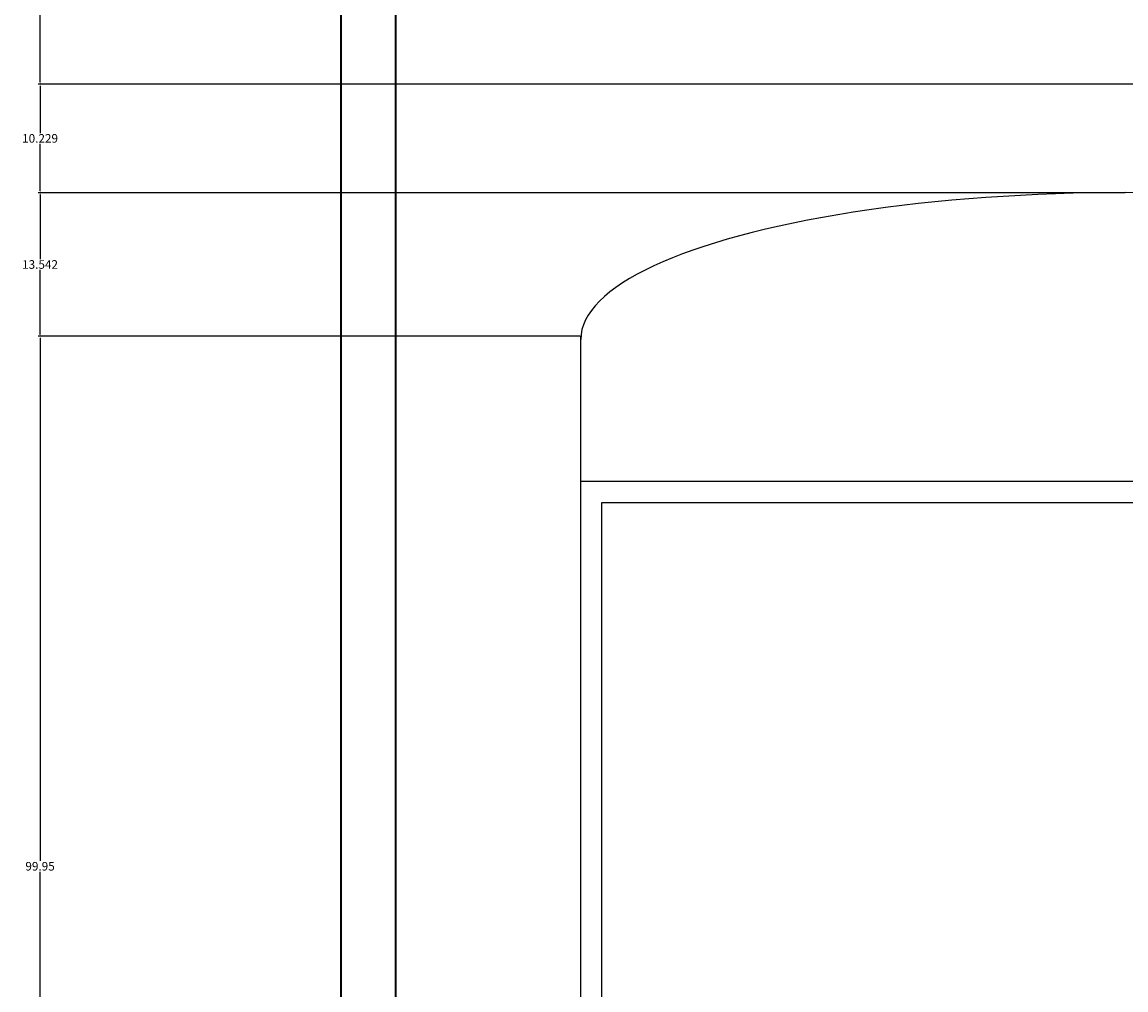
# Model space of a CAD drawing. Units: inches. Extents: x 69 to 650, y -16 to 573.
# Tile 2 of 26: x 69 to 174, y 126 to 218. Entities that reach past the tile are written whole.
import ezdxf

# ---------------------------------------------------------------- set-up
doc = ezdxf.new("R2010")
doc.units = ezdxf.units.IN
doc.header["$MEASUREMENT"] = 0
for name, color, linetype, lineweight in [('A-ANNO-DIMS', 2, 'Continuous', 18), ('A-DOOR', 3, 'Continuous', 25), ('A-WALL', 7, 'Continuous', 35)]:
    doc.layers.add(name, color=color, linetype=linetype, lineweight=lineweight)
doc.styles.get("Standard").update_dxf_attribs({"font": 'arial.ttf'})
doc.dimstyles.get("Standard").update_dxf_attribs({"dimtxt": 0.8125, "dimasz": 0.18, "dimexe": 0.18, "dimexo": 0.0625, "dimgap": 0.09, "dimtad": 0, "dimtih": 1, "dimtoh": 1, "dimdec": 4, "dimzin": 0, "dimdsep": 46, "dimlunit": 4, "dimtxsty": 'Standard', "dimcen": 0.09, "dimadec": 0, "dimazin": 0, "dimtfac": 1, "dimtdec": 4, "dimtofl": 0, "dimtmove": 0, "dimatfit": 3, "dimfxl": 1, "dimtolj": 1, "dimtzin": 0, "dimarcsym": 0})

# ---------------------------------------------------------------- blocks, each defined once
blk = doc.blocks.new('*D19')
at = {"layer": 'A-ANNO-DIMS', "color": 0, "lineweight": -2, "transparency": 16777216}
for p, q in [((99.56, 471.72), (99.56, 572.74)), ((619.56, 87.99), (619.56, 572.74)), ((99.74, 572.56), (358.57, 572.56)), ((619.38, 572.56), (360.54, 572.56))]:
    blk.add_line(p, q, dxfattribs=at)
at = {"layer": 'A-ANNO-DIMS', "color": 0, "transparency": 16777216}
for points in [[(99.74, 572.59), (99.74, 572.53), (99.56, 572.56)], [(619.38, 572.59), (619.38, 572.53), (619.56, 572.56)]]:
    blk.add_solid(points, dxfattribs=at)
at = {"layer": 'Defpoints', "color": 0, "transparency": 16777216}
for p in [(619.56, 572.56), (99.56, 471.66), (619.56, 87.93)]:
    blk.add_point(p, dxfattribs=at)
at = {"layer": 'A-ANNO-DIMS', "color": 0, "transparency": 16777216, "insert": (359.56, 572.56), "char_height": 0.812, "attachment_point": 5}
blk.add_mtext('\\A1;520', dxfattribs=at)
blk = doc.blocks.new('*D22')
at = {"layer": 'A-ANNO-DIMS', "color": 0, "lineweight": -2, "transparency": 16777216}
for p, q in [((122.09, 187.88), (70.98, 187.88)), ((71.16, 187.7), (71.16, 138.41)), ((71.16, 88.11), (71.16, 137.4)), ((122.09, 87.93), (70.98, 87.93))]:
    blk.add_line(p, q, dxfattribs=at)
at = {"layer": 'A-ANNO-DIMS', "color": 0, "transparency": 16777216}
for points in [[(71.13, 187.7), (71.19, 187.7), (71.16, 187.88)], [(71.13, 88.11), (71.19, 88.11), (71.16, 87.93)]]:
    blk.add_solid(points, dxfattribs=at)
at = {"layer": 'Defpoints', "color": 0, "transparency": 16777216}
for p in [(71.16, 187.88), (122.16, 187.88), (122.16, 87.93)]:
    blk.add_point(p, dxfattribs=at)
at = {"layer": 'A-ANNO-DIMS', "color": 0, "transparency": 16777216, "insert": (71.16, 137.91), "char_height": 0.812, "attachment_point": 5}
blk.add_mtext('\\A1;99.95', dxfattribs=at)
blk = doc.blocks.new('*D23')
at = {"layer": 'A-ANNO-DIMS', "color": 0, "lineweight": -2, "transparency": 16777216}
for p, q in [((173.51, 201.42), (70.98, 201.42)), ((71.16, 201.24), (71.16, 195.16)), ((71.16, 188.06), (71.16, 194.15)), ((122.09, 187.88), (70.98, 187.88))]:
    blk.add_line(p, q, dxfattribs=at)
at = {"layer": 'A-ANNO-DIMS', "color": 0, "transparency": 16777216}
for points in [[(71.13, 201.24), (71.19, 201.24), (71.16, 201.42)], [(71.13, 188.06), (71.19, 188.06), (71.16, 187.88)]]:
    blk.add_solid(points, dxfattribs=at)
at = {"layer": 'Defpoints', "color": 0, "transparency": 16777216}
for p in [(71.16, 201.42), (173.58, 201.42), (122.16, 187.88)]:
    blk.add_point(p, dxfattribs=at)
at = {"layer": 'A-ANNO-DIMS', "color": 0, "transparency": 16777216, "insert": (71.16, 194.65), "char_height": 0.812, "attachment_point": 5}
blk.add_mtext('\\A1;13.542', dxfattribs=at)
blk = doc.blocks.new('*D24')
at = {"layer": 'A-ANNO-DIMS', "color": 0, "lineweight": -2, "transparency": 16777216}
for p, q in [((441.88, 211.65), (70.98, 211.65)), ((71.16, 211.47), (71.16, 207.04)), ((71.16, 201.6), (71.16, 206.03)), ((173.51, 201.42), (70.98, 201.42))]:
    blk.add_line(p, q, dxfattribs=at)
at = {"layer": 'A-ANNO-DIMS', "color": 0, "transparency": 16777216}
for points in [[(71.13, 211.47), (71.19, 211.47), (71.16, 211.65)], [(71.13, 201.6), (71.19, 201.6), (71.16, 201.42)]]:
    blk.add_solid(points, dxfattribs=at)
at = {"layer": 'Defpoints', "color": 0, "transparency": 16777216}
for p in [(71.16, 211.65), (441.94, 211.65), (173.58, 201.42)]:
    blk.add_point(p, dxfattribs=at)
at = {"layer": 'A-ANNO-DIMS', "color": 0, "transparency": 16777216, "insert": (71.16, 206.54), "char_height": 0.812, "attachment_point": 5}
blk.add_mtext('\\A1;10.229', dxfattribs=at)
blk = doc.blocks.new('*D25')
at = {"layer": 'A-ANNO-DIMS', "color": 0, "lineweight": -2, "transparency": 16777216}
for p, q in [((99.49, 243.93), (70.98, 243.93)), ((71.16, 243.75), (71.16, 228.3)), ((71.16, 211.83), (71.16, 227.29)), ((441.88, 211.65), (70.98, 211.65))]:
    blk.add_line(p, q, dxfattribs=at)
at = {"layer": 'A-ANNO-DIMS', "color": 0, "transparency": 16777216}
for points in [[(71.13, 243.75), (71.19, 243.75), (71.16, 243.93)], [(71.13, 211.83), (71.19, 211.83), (71.16, 211.65)]]:
    blk.add_solid(points, dxfattribs=at)
at = {"layer": 'Defpoints', "color": 0, "transparency": 16777216}
for p in [(71.16, 243.93), (99.56, 243.93), (441.94, 211.65)]:
    blk.add_point(p, dxfattribs=at)
at = {"layer": 'A-ANNO-DIMS', "color": 0, "transparency": 16777216, "insert": (71.16, 227.79), "char_height": 0.812, "attachment_point": 5}
blk.add_mtext('\\A1;32.28', dxfattribs=at)
blk = doc.blocks.new('*D35')
at = {"layer": 'A-ANNO-DIMS', "color": 0, "lineweight": -2, "transparency": 16777216}
for p, q in [((99.56, 243.87), (99.56, 35.35)), ((190.3, 243.87), (190.3, 35.35)), ((99.74, 35.53), (143.47, 35.53)), ((190.12, 35.53), (146.39, 35.53))]:
    blk.add_line(p, q, dxfattribs=at)
at = {"layer": 'A-ANNO-DIMS', "color": 0, "transparency": 16777216}
for points in [[(99.74, 35.56), (99.74, 35.5), (99.56, 35.53)], [(190.12, 35.56), (190.12, 35.5), (190.3, 35.53)]]:
    blk.add_solid(points, dxfattribs=at)
at = {"layer": 'Defpoints', "color": 0, "transparency": 16777216}
for p in [(99.56, 243.93), (190.3, 243.93), (190.3, 35.53)]:
    blk.add_point(p, dxfattribs=at)
at = {"layer": 'A-ANNO-DIMS', "color": 0, "transparency": 16777216, "insert": (144.93, 35.53), "char_height": 0.812, "attachment_point": 5}
blk.add_mtext('\\A1;90.74', dxfattribs=at)

msp = doc.modelspace()

# ---------------------------------------------------------------- linework, layer by layer
at = {"layer": 'A-DOOR'}
msp.add_line((122.1565, 174.2116), (122.1565, 187.8805), dxfattribs=at)
for points in [[(122.1565, 174.2116), (224.9972, 174.2116), (224.9972, 87.93), (122.1565, 87.93)], [(124.1565, 172.2116), (222.9972, 172.2116), (222.9972, 89.93), (124.1565, 89.93)]]:
    msp.add_lwpolyline(points, close=True, dxfattribs=at)
msp.add_ellipse((173.5769, 187.5726), major_axis=(-51.4203, 0.0194), ratio=0.26935388, start_param=3.14159265, end_param=6.28338858, dxfattribs=at)
at = {"layer": 'A-WALL'}
for p, q in [((99.556, 87.93), (99.556, 231.93)), ((104.6982, 231.93), (104.6982, 87.93))]:
    msp.add_line(p, q, dxfattribs=at)

# ---------------------------------------------------------------- dimensions: what is measured, and where the dimension line sits
at = {"layer": 'A-ANNO-DIMS'}
for base, p1, p2, override, picture, middle in [((619.555, 572.5573), (99.556, 471.6595), (619.555, 87.93), {"dimdec": 0, "dimlfac": 1, "dimrnd": 0, "dimzin": 0, "dimdsep": 46, "dimlunit": 2}, '*D19', (359.5555, 572.5573)), ((190.299, 35.53), (99.556, 243.93), (190.299, 243.93), {"dimdec": 2, "dimlfac": 1, "dimrnd": 0, "dimzin": 0, "dimdsep": 46, "dimlunit": 2}, '*D35', (144.9275, 35.53))]:
    dim = msp.add_linear_dim(base=base, p1=p1, p2=p2, dimstyle='Standard', override=override, dxfattribs=at)
    dim.commit()
    dim.dimension.update_dxf_attribs({"geometry": picture, "text_midpoint": middle})
for base, p1, p2, override, picture, middle in [((71.156, 243.93), (441.9398, 211.6519), (99.556, 243.93), {"dimdec": 2, "dimlfac": 1, "dimrnd": 0, "dimzin": 0, "dimdsep": 46, "dimlunit": 2}, '*D25', (71.156, 227.7909)), ((71.156, 211.6519), (173.5769, 201.4229), (441.9398, 211.6519), {"dimdec": 3, "dimlfac": 1, "dimrnd": 0, "dimzin": 0, "dimdsep": 46, "dimlunit": 2}, '*D24', (71.156, 206.5374)), ((71.156, 201.4229), (122.1565, 187.8805), (173.5769, 201.4229), {"dimdec": 3, "dimlfac": 1, "dimrnd": 0, "dimzin": 0, "dimdsep": 46, "dimlunit": 2}, '*D23', (71.156, 194.6517)), ((71.156, 187.8805), (122.1565, 87.93), (122.1565, 187.8805), {"dimdec": 2, "dimlfac": 1, "dimrnd": 0, "dimzin": 0, "dimdsep": 46, "dimlunit": 2}, '*D22', (71.156, 137.9053))]:
    dim = msp.add_linear_dim(base=base, p1=p1, p2=p2, angle=90, dimstyle='Standard', override=override, dxfattribs=at)
    dim.commit()
    dim.dimension.update_dxf_attribs({"geometry": picture, "text_midpoint": middle})

doc.saveas('drawing.dxf')
